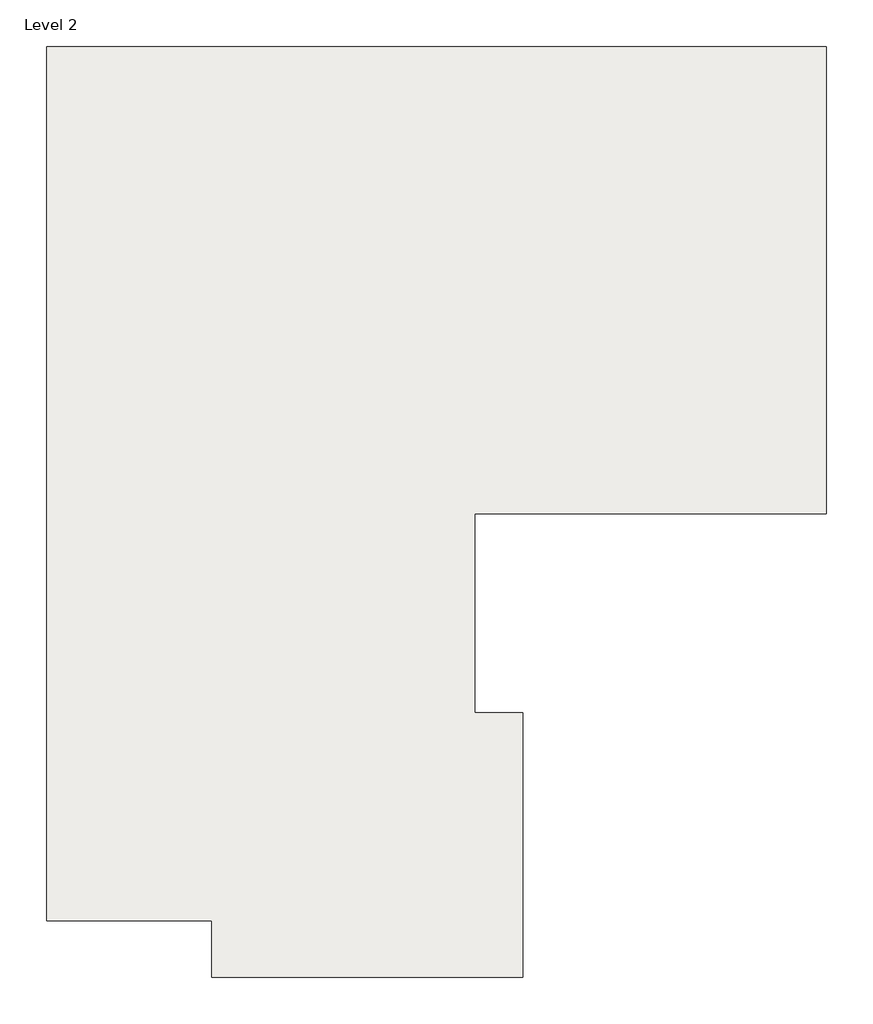
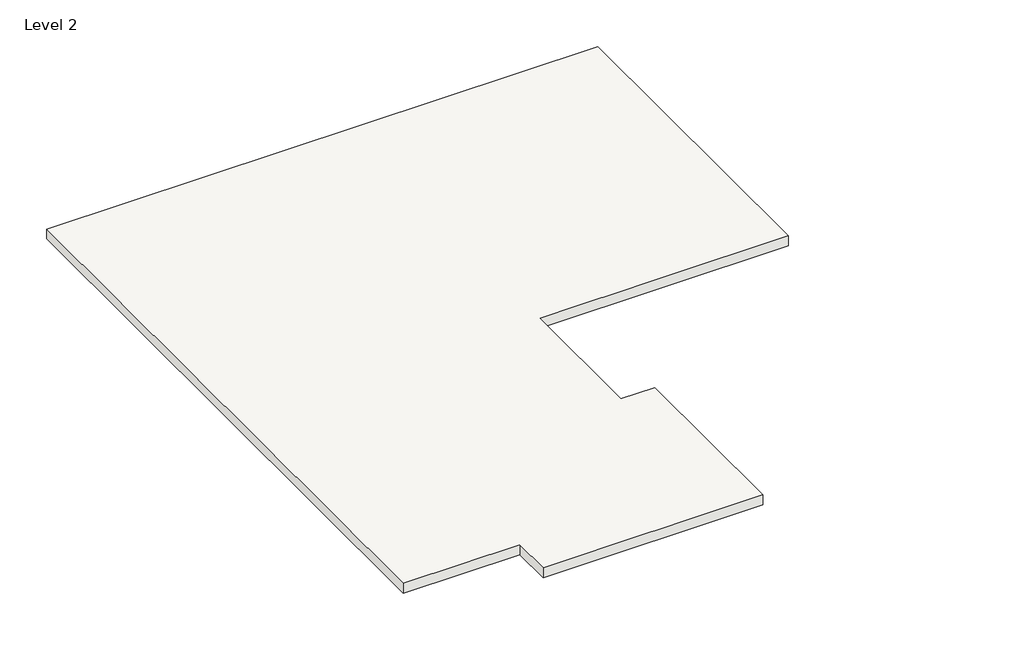
# One storey: 1 roof.
"""IFC4 building model written with IfcOpenShell, lengths in millimetres."""

from ifc_helpers import new_model, si_unit, frame, origin, place, context, project, spatial, polyline, outline, extrude, element, save

model = new_model("IFC4")

# Units and contexts
model_context = context("Model", 3, world=origin())
ifc_project = project(units=[si_unit("LENGTHUNIT", "METRE", prefix="MILLI")], contexts=[model_context])

# Site, building, storey
site = spatial("IfcSite", under=ifc_project)
building = spatial("IfcBuilding", under=site)
storey = spatial("IfcBuildingStorey", under=building, Name="Level 2", Elevation=3048.0)

# Roof
placement = place(None, origin())
element("IfcRoof", 1, ObjectType="Wood Rafter 8\" - Asphalt Shingle - Insulated", at=placement, inside=storey, context=model_context, shape_type="SweptSolid", body=[
    extrude(outline(polyline([(-11739.7886283, 11933.9574946), (-589.1886283, 11933.9574946), (-589.1886283, 5253.7574946), (-5618.3886283, 5253.7574946), (-5618.3886283, 2408.9574946), (-4932.5886283, 2408.9574946), (-4932.5886283, -1375.6425054), (-9377.5886283, -1375.6425054), (-9377.5886283, -562.8425054), (-11739.7886283, -562.8425054), (-11739.7886283, 11933.9574946)])), frame((0.0, 0.0, 3048.0), z_axis=(0.0, 0.0, 1.0), x_axis=(1.0, 0.0, 0.0)), (0.0, 0.0, 1.0), 212.725),
])

save(model, "model.ifc")

# Revit data of these elements
# Type "Wood Rafter 8\" - Asphalt Shingle - Insulated"
#   Assembly Code = "B1020"
#   Layers, outside or top first: 0' - 0 1/4" "Asphalt Shingle" (function 4); 0' - 0 5/8" "Plywood, Sheathing" (function 2); 0' - 7 1/2" "Structure, Wood Joist/Rafter Layer, Batt Insulation" (function 1)
# Element 1 (IfcRoof, "Wood Rafter 8\" - Asphalt Shingle - Insulated")
#   built-in parameter 1001705 = 10.6979 (stored number, unit not read)
#   built-in parameter 1001710 = 33615
#   Phase Created = New Construction
#   Materials on its faces: "Structure, Wood Joist/Rafter Layer, Batt Insulation", "Asphalt Shingle"
# Materials
#   "Asphalt Shingle": class "Generic", colour RGB 155 155 155, transparency 0, Description = "Asphalt roofing shingle", Cost = 0
#   "Plywood, Sheathing": class "Wood", colour RGB 212 179 113, transparency 0, Description = "Plywood, sheathing grade", Cost = 0
#   "Structure, Wood Joist/Rafter Layer, Batt Insulation": class "Wood", colour RGB 127 127 127, transparency 0, Description = "Wood framing, insulated", Cost = 0
